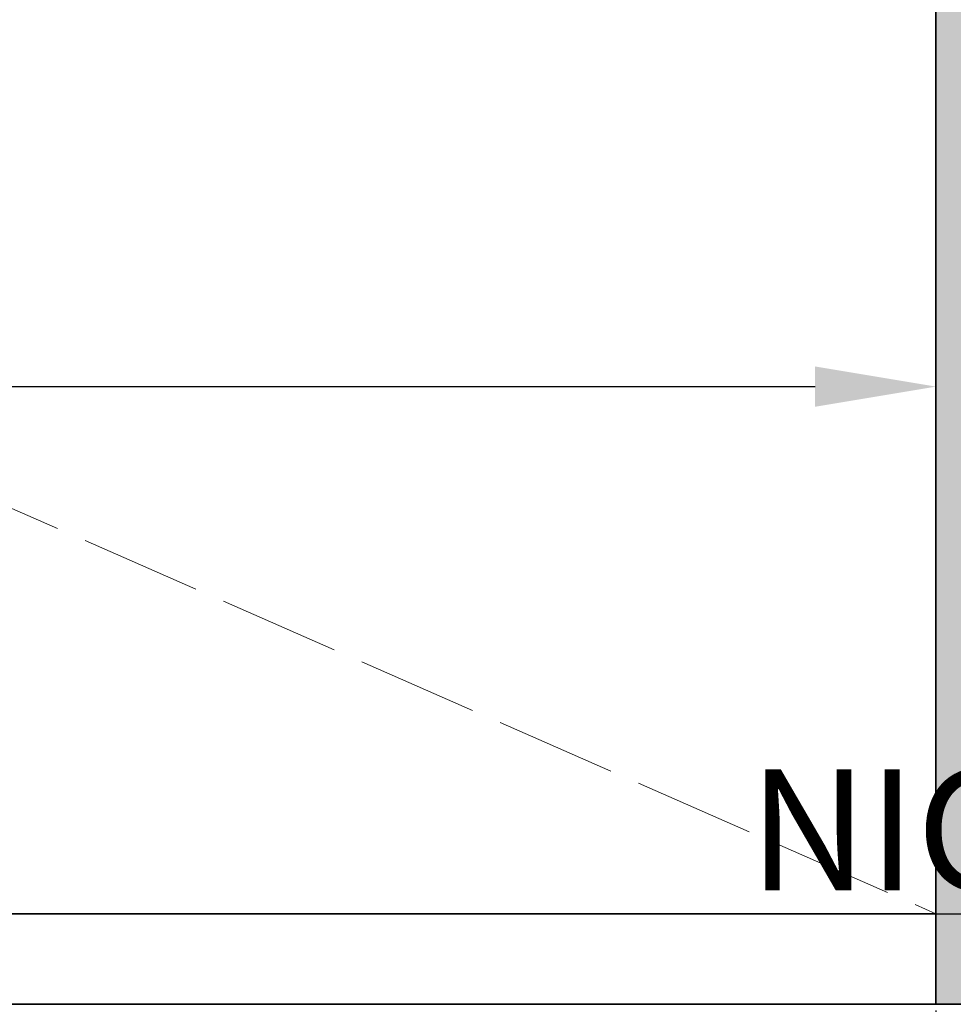
# Model space of a CAD drawing. Units: inches. Extents: x 2083 to 3317, y 1141 to 2115.
# Tile 110 of 256: x 2772 to 2865, y 1263 to 1361. Entities that reach past the tile are written whole.
import ezdxf

# ---------------------------------------------------------------- set-up
doc = ezdxf.new("R2010")
doc.units = ezdxf.units.IN
doc.linetypes.add('ACAD_ISO02W100', pattern=[15, 12, -3])
for name, color, linetype, lineweight in [('A-ANNO-DIMS', 2, 'Continuous', 18), ('A-FLOR-OPEN', 8, 'ACAD_ISO02W100', 13), ('A-WALL', 7, 'Continuous', 35)]:
    doc.layers.add(name, color=color, linetype=linetype, lineweight=lineweight)
doc.layers.add('A-WALL-PATT', color=251, linetype='Continuous', lineweight=13, true_color=0x636466)
doc.styles.get("Standard").update_dxf_attribs({"font": 'arial.ttf'})
doc.dimstyles.new('ISO-25', dxfattribs={"dimtxt": 12, "dimasz": 12, "dimexe": 1.25, "dimexo": 0.625, "dimtad": 1, "dimlunit": 3, "dimtxsty": 'Standard', "dimcen": 2.5, "dimadec": 0, "dimazin": 0, "dimtfac": 1, "dimtmove": 0, "dimatfit": 3, "dimfxl": 1, "dimarcsym": 0})

# ---------------------------------------------------------------- blocks, each defined once
blk = doc.blocks.new('*D10')
at = {"layer": 'A-ANNO-DIMS', "color": 0, "lineweight": -2, "transparency": 16777216}
for p, q in [((2862.96, 1262.636), (2862.96, 1201.384)), ((3126.96, 1262.636), (3126.96, 1201.384)), ((2874.96, 1202.634), (3114.96, 1202.634))]:
    blk.add_line(p, q, dxfattribs=at)
at = {"layer": 'A-ANNO-DIMS', "color": 0, "transparency": 16777216}
for points in [[(2874.96, 1204.634), (2874.96, 1200.634), (2862.96, 1202.634)], [(3114.96, 1204.634), (3114.96, 1200.634), (3126.96, 1202.634)]]:
    blk.add_solid(points, dxfattribs=at)
at = {"layer": 'Defpoints', "color": 0, "transparency": 16777216}
for p in [(2862.96, 1263.261), (3126.96, 1263.261), (3126.96, 1202.634)]:
    blk.add_point(p, dxfattribs=at)
at = {"layer": 'A-ANNO-DIMS', "color": 0, "transparency": 16777216, "insert": (2994.96, 1209.284), "char_height": 12, "attachment_point": 5}
blk.add_mtext("22'", dxfattribs=at)
blk = doc.blocks.new('*D11')
at = {"layer": 'A-ANNO-DIMS', "color": 0, "lineweight": -2, "transparency": 16777216}
for p, q in [((2544.96, 1262.636), (2544.96, 1201.284)), ((2862.96, 1262.636), (2862.96, 1201.284)), ((2556.96, 1202.534), (2850.96, 1202.534))]:
    blk.add_line(p, q, dxfattribs=at)
at = {"layer": 'A-ANNO-DIMS', "color": 0, "transparency": 16777216}
for points in [[(2556.96, 1204.534), (2556.96, 1200.534), (2544.96, 1202.534)], [(2850.96, 1204.534), (2850.96, 1200.534), (2862.96, 1202.534)]]:
    blk.add_solid(points, dxfattribs=at)
at = {"layer": 'Defpoints', "color": 0, "transparency": 16777216}
for p in [(2544.96, 1263.261), (2862.96, 1263.261), (2862.96, 1202.534)]:
    blk.add_point(p, dxfattribs=at)
at = {"layer": 'A-ANNO-DIMS', "color": 0, "transparency": 16777216, "insert": (2703.96, 1209.286), "char_height": 12, "attachment_point": 5}
blk.add_mtext('26\'-6"', dxfattribs=at)
blk = doc.blocks.new('*D26')
at = {"layer": 'A-ANNO-DIMS', "color": 0, "lineweight": -2, "transparency": 16777216}
for p, q in [((3088.986, 1274.915), (3088.986, 1270.952)), ((3111.24, 1274.915), (3111.24, 1270.952)), ((3076.986, 1272.202), (2840.262, 1272.202)), ((3111.24, 1272.202), (3088.986, 1272.202)), ((3123.24, 1272.202), (3135.24, 1272.202))]:
    blk.add_line(p, q, dxfattribs=at)
at = {"layer": 'A-ANNO-DIMS', "color": 0, "transparency": 16777216}
for points in [[(3076.986, 1274.202), (3076.986, 1270.202), (3088.986, 1272.202)], [(3123.24, 1274.202), (3123.24, 1270.202), (3111.24, 1272.202)]]:
    blk.add_solid(points, dxfattribs=at)
at = {"layer": 'Defpoints', "color": 0, "transparency": 16777216}
for p in [(3088.986, 1275.54), (3111.24, 1275.54), (3088.986, 1272.202)]:
    blk.add_point(p, dxfattribs=at)
at = {"layer": 'A-ANNO-DIMS', "color": 0, "transparency": 16777216, "insert": (2952.624, 1279.032), "char_height": 12, "attachment_point": 5}
blk.add_mtext('NIGHTSTAND 1\'-10 1/2" TYP.', dxfattribs=at)
blk = doc.blocks.new('*D66')
at = {"layer": 'A-ANNO-DIMS', "color": 0, "lineweight": -2, "transparency": 16777216}
for p, q in [((2544.96, 1272.886), (2544.96, 1325.861)), ((2862.96, 1272.886), (2862.96, 1325.861)), ((2556.96, 1324.611), (2850.96, 1324.611))]:
    blk.add_line(p, q, dxfattribs=at)
at = {"layer": 'A-ANNO-DIMS', "color": 0, "transparency": 16777216}
for points in [[(2556.96, 1326.611), (2556.96, 1322.611), (2544.96, 1324.611)], [(2850.96, 1326.611), (2850.96, 1322.611), (2862.96, 1324.611)]]:
    blk.add_solid(points, dxfattribs=at)
at = {"layer": 'Defpoints', "color": 0, "transparency": 16777216}
for p in [(2862.96, 1324.611), (2544.96, 1272.261), (2862.96, 1272.261)]:
    blk.add_point(p, dxfattribs=at)
at = {"layer": 'A-ANNO-DIMS', "color": 0, "transparency": 16777216, "insert": (2703.96, 1331.363), "char_height": 12, "attachment_point": 5}
blk.add_mtext('26\'-6"', dxfattribs=at)

msp = doc.modelspace()

# ---------------------------------------------------------------- hatches: boundary and pattern name
at = {"layer": 'A-WALL-PATT'}
h = msp.add_hatch(color=256, dxfattribs=at)
h.dxf.hatch_style = 1
h.paths.add_polyline_path([(3126.96, 2020.761), (2748.96, 2020.761), (2604.96, 2020.761), (2226.96, 2020.761), (2226.96, 1702.761), (2466.96, 1702.761), (2466.96, 1582.761), (2418.96, 1582.761), (2418.96, 1477.761), (2226.96, 1477.761), (2226.96, 1263.261), (2544.96, 1263.261), (2544.96, 1411.761), (2604.96, 1411.761), (2685.96, 1411.761), (2685.96, 1420.761), (2604.96, 1420.761), (2604.96, 1573.761), (2604.96, 1702.761), (2604.96, 2011.761), (2748.96, 2011.761), (2748.96, 1702.761), (2862.96, 1702.761), (2862.96, 1621.761), (2871.96, 1621.761), (2871.96, 1702.761), (2883.96, 1702.761), (2883.96, 1706.939, -0.026459), (2883.96, 1711.761), (2757.96, 1711.761), (2757.96, 1807.761), (2787.96, 1807.761), (2787.96, 1812.261), (2757.96, 1812.261), (2757.96, 2011.761), (2877.96, 2011.761), (2877.96, 1812.261), (2847.96, 1812.261), (2847.96, 1807.761), (2889.836, 1807.761), (2889.836, 1812.261), (2882.46, 1812.261), (2882.46, 2011.761), (3117.96, 2011.761), (3117.96, 1812.261), (2937.836, 1812.261), (2937.836, 1807.761), (2995.71, 1807.761), (2995.71, 1796.118), (3000.21, 1796.118), (3000.21, 1807.761), (3117.96, 1807.761), (3117.96, 1711.761), (3000.21, 1711.761), (3000.21, 1760.118), (2998.573, 1760.118, -0.020711), (2995.71, 1760.118), (2995.71, 1711.761), (2931.96, 1711.761), (2931.96, 1702.761), (3126.96, 1702.761)])
h.paths.add_polyline_path([(2471.46, 2011.761), (2471.46, 1810.011), (2462.717, 1810.011), (2462.717, 1805.511), (2505.96, 1805.511), (2505.96, 1810.011), (2475.96, 1810.011), (2475.96, 2011.761), (2595.96, 2011.761), (2595.96, 1810.011), (2565.96, 1810.011), (2565.96, 1805.511), (2595.96, 1805.511), (2595.96, 1711.761), (2235.96, 1711.761), (2235.96, 1805.511), (2353.71, 1805.511), (2353.71, 1796.054), (2358.21, 1796.054), (2358.21, 1805.511), (2414.717, 1805.511), (2414.717, 1810.011), (2235.96, 1810.011), (2235.96, 2011.761)], flags=16)
h.paths.add_polyline_path([(2270.205, 1994.61), (2270.205, 1970.61), (2246.205, 1970.61), (2246.205, 1994.61)], flags=0)
edge = h.paths.add_edge_path(flags=0)
edge.add_ellipse((2332.027, 1899.798), major_axis=(-3.043, 3.043), ratio=0.168252, start_angle=-161.33217, end_angle=-156.30711, ccw=False)
edge.add_ellipse((2333.082, 1898.744), major_axis=(-1.055, 1.055), ratio=0.453532, start_angle=-123.37102, end_angle=-94.15911)
edge = h.paths.add_edge_path(flags=0)
edge.add_ellipse((2332.027, 1968.876), major_axis=(3.043, 3.043), ratio=0.168252, start_angle=18.66783, end_angle=23.69289)
edge.add_spline(control_points=[(2332.926, 1970.691), (2332.227, 1970.336), (2330.894, 1969.659), (2328.413, 1970.932), (2327.204, 1967.749), (2324.71, 1969.956), (2322.533, 1967.012), (2320.013, 1971.296), (2317.68, 1968.158), (2316.041, 1967.102), (2315.427, 1966.81)], knot_values=[0, 0, 0, 0, 2.267059, 4.324559, 6.685584, 8.878641, 11.121502, 14.300359, 17.755284, 19.732645, 19.732645, 19.732645, 19.732645], degree=3, periodic=0)
edge.add_ellipse((2332.027, 1968.876), major_axis=(3.043, 3.043), ratio=0.168252, start_angle=18.66783, end_angle=23.69289, ccw=False)
edge.add_ellipse((2333.082, 1969.931), major_axis=(1.055, 1.055), ratio=0.453532, start_angle=56.62898, end_angle=85.84089, ccw=False)
edge = h.paths.add_edge_path(flags=0)
edge.add_spline(control_points=[(2296.428, 1967.988), (2293.628, 1965.336), (2287.704, 1959.727), (2299.744, 1949.996), (2294.533, 1935.669), (2290.573, 1920.604), (2293.394, 1909.974), (2296.185, 1904.967)], knot_values=[0.099185, 0.099185, 0.099185, 0.099185, 0.345301, 0.619822, 0.982653, 1.386093, 1.810555, 1.810555, 1.810555, 1.810555], degree=3, periodic=0)
edge.add_spline(control_points=[(2296.185, 1904.967), (2297.384, 1902.619), (2298.001, 1901.949), (2298.553, 1901.468)], knot_values=[0.006246, 0.006246, 0.006246, 0.006246, 0.055476, 0.055476, 0.055476, 0.055476], degree=3, periodic=0)
edge.add_spline(control_points=[(2298.553, 1901.468), (2297.259, 1900.923), (2295.225, 1900.232), (2293.06, 1900.614), (2292.101, 1900.788), (2292.09, 1900.791)], knot_values=[0.312835, 0.312835, 0.312835, 0.312835, 0.40178, 0.474987, 0.475903, 0.475903, 0.475903, 0.475903], degree=3, periodic=0)
edge.add_arc((2292.794, 1904.664), 3.937, 215.4209, 259.69818, ccw=False)
edge.add_spline(control_points=[(2289.585, 1902.382), (2289.477, 1902.535), (2289.368, 1902.688), (2289.261, 1902.841)], knot_values=[0.102872, 0.102872, 0.102872, 0.102872, 0.116896, 0.116896, 0.116896, 0.116896], degree=3, periodic=0)
edge.add_spline(control_points=[(2289.261, 1902.841), (2288.687, 1902.55), (2287.64, 1902.02), (2285.881, 1901.874), (2283.853, 1901.504), (2281.72, 1899.711), (2278.467, 1899.493), (2276.157, 1901.883), (2272.259, 1899.804), (2267.778, 1901.843), (2262.244, 1900.184), (2257.415, 1901.782), (2254.318, 1900.726), (2253.178, 1900.337)], knot_values=[0, 0, 0, 0, 1.907977, 3.477176, 5.261074, 7.972851, 11.680248, 13.717921, 16.939592, 22.789562, 27.502503, 33.595215, 37.145618, 37.145618, 37.145618, 37.145618], degree=3, periodic=0)
edge.add_line((2253.178, 1900.337), (2250.244, 1902.841))
edge.add_line((2250.244, 1902.841), (2250.244, 1965.833))
edge.add_line((2250.244, 1965.833), (2253.178, 1968.337))
edge.add_spline(control_points=[(2253.178, 1968.337), (2254.318, 1967.948), (2257.415, 1966.892), (2262.244, 1968.49), (2267.778, 1966.831), (2271.527, 1968.537), (2273.876, 1967.828), (2274.207, 1967.728)], knot_values=[0, 0, 0, 0, 0.09018, 0.244935, 0.364644, 0.513233, 0.537855, 0.537855, 0.537855, 0.537855], degree=3, periodic=0)
edge.add_arc((2274.353, 1963.793), 3.937, 72.05113, 92.12795, ccw=False)
edge.add_arc((2281.297, 1985.23), 18.596, 252.05113, 288.56572)
edge.add_arc((2292.317, 1956.029), 12.646, 71.02679, 113.77822, ccw=False)
edge = h.paths.add_edge_path(flags=0)
edge.add_spline(control_points=[(2274.899, 1951.856), (2275.066, 1951.617), (2275.233, 1951.377), (2275.398, 1951.136)], knot_values=[1.409916, 1.409916, 1.409916, 1.409916, 1.43159, 1.43159, 1.43159, 1.43159], degree=3, periodic=0)
edge.add_spline(control_points=[(2275.398, 1951.136), (2275.792, 1950.562), (2276.179, 1949.984), (2276.546, 1949.397)], knot_values=[1.358238, 1.358238, 1.358238, 1.358238, 1.409916, 1.409916, 1.409916, 1.409916], degree=3, periodic=0)
edge.add_line((2276.546, 1949.397), (2277.437, 1947.862))
edge.add_spline(control_points=[(2277.437, 1947.862), (2276.304, 1945.673), (2274.64, 1942.427), (2274.632, 1938.094), (2272.799, 1930.852), (2274.356, 1943.897), (2275.948, 1947.923), (2276.546, 1949.397)], knot_values=[0.005632, 0.005632, 0.005632, 0.005632, 0.186014, 0.266002, 0.357087, 0.59639, 0.739732, 0.739732, 0.739732, 0.739732], degree=3, periodic=0)
edge.add_spline(control_points=[(2276.546, 1949.397), (2276.179, 1949.984), (2275.792, 1950.562), (2275.398, 1951.136)], knot_values=[1.358238, 1.358238, 1.358238, 1.358238, 1.409916, 1.409916, 1.409916, 1.409916], degree=3, periodic=0)
edge.add_spline(control_points=[(2275.398, 1951.136), (2274.943, 1950.08), (2274.208, 1948.025), (2273.935, 1944.851), (2272.469, 1937.627), (2273.466, 1945.696), (2274.701, 1951.059), (2274.899, 1951.856)], knot_values=[0.104364, 0.104364, 0.104364, 0.104364, 0.189636, 0.269624, 0.36071, 0.600013, 0.644622, 0.644622, 0.644622, 0.644622], degree=3, periodic=0)
h.paths.add_polyline_path([(2269.168, 1963.128, -0.357527), (2268.171, 1960.976, -0.092561), (2268.171, 1939.436, -0.357527), (2269.168, 1937.285, -0.357527), (2267.016, 1938.282, -0.164785), (2254.686, 1938.282, -0.357527), (2252.534, 1937.285, -0.357527), (2253.531, 1939.436, -0.092561), (2253.531, 1960.976, -0.357527), (2252.534, 1963.128, -0.357527), (2254.686, 1962.131, -0.164785), (2267.016, 1962.131, -0.357527)], flags=0)
h.paths.add_polyline_path([(2248.874, 1967.802), (2248.874, 1957.028), (2249.458, 1957.028), (2249.458, 1911.647), (2248.874, 1911.647), (2248.874, 1900.873), (2246.512, 1900.873, 0.197327), (2244.15, 1902.457), (2244.15, 1966.218, 0.197327), (2246.512, 1967.802)], flags=0)
h.paths.add_polyline_path([(2269.168, 1931.389, -0.357527), (2268.171, 1929.238, -0.092561), (2268.171, 1907.698, -0.357527), (2269.168, 1905.547, -0.357527), (2267.016, 1906.544, -0.164785), (2254.686, 1906.544, -0.357527), (2252.534, 1905.547, -0.357527), (2253.531, 1907.698, -0.092561), (2253.531, 1929.238, -0.357527), (2252.534, 1931.389, -0.357527), (2254.686, 1930.392, -0.164785), (2267.016, 1930.392, -0.357527)], flags=0)
edge = h.paths.add_edge_path(flags=0)
edge.add_spline(control_points=[(2276.197, 1906.724), (2276.168, 1909.029), (2276.114, 1913.372), (2270.598, 1924.925), (2273.905, 1919.013), (2275.922, 1916.262), (2275.475, 1912.402), (2277.258, 1910.381), (2276.696, 1908.225), (2276.646, 1906.813), (2276.618, 1906.008)], knot_values=[0, 0, 0, 0, 8.61026, 16.221274, 18.843057, 23.804898, 27.440828, 29.356102, 31.203478, 33.650687, 33.650687, 33.650687, 33.650687], degree=3, periodic=0)
edge.add_spline(control_points=[(2276.618, 1906.008), (2276.623, 1905.624), (2276.498, 1904.629), (2275.442, 1903.855), (2274.937, 1903.08), (2274.859, 1902.841)], knot_values=[0.156488, 0.156488, 0.156488, 0.156488, 0.184398, 0.231376, 0.250598, 0.250598, 0.250598, 0.250598], degree=3, periodic=0)
edge.add_line((2274.859, 1902.841), (2276.506, 1902.841))
edge.add_spline(control_points=[(2276.506, 1902.841), (2276.788, 1903.085), (2277.665, 1904.125), (2278.25, 1904.341), (2277.654, 1908.527), (2278.156, 1906.228), (2278.1, 1905.286), (2278.847, 1904.069), (2277.857, 1903.415), (2277.874, 1902.991), (2277.904, 1902.841)], knot_values=[0.059574, 0.059574, 0.059574, 0.059574, 0.080753, 0.103741, 0.16972, 0.176036, 0.207137, 0.240474, 0.262341, 0.27366, 0.27366, 0.27366, 0.27366], degree=3, periodic=0)
edge.add_line((2277.904, 1902.841), (2280.03, 1902.841))
edge.add_spline(control_points=[(2280.03, 1902.841), (2279.888, 1903.088), (2279.499, 1903.982), (2280.152, 1905.939), (2278.104, 1909.658), (2279.762, 1907.185), (2280.328, 1904.875), (2280.485, 1903.49), (2281.463, 1903.249), (2281.758, 1902.936), (2281.834, 1902.841)], knot_values=[0.013856, 0.013856, 0.013856, 0.013856, 0.034874, 0.088867, 0.107879, 0.126738, 0.158714, 0.193757, 0.217487, 0.226722, 0.226722, 0.226722, 0.226722], degree=3, periodic=0)
edge.add_spline(control_points=[(2281.834, 1902.841), (2281.788, 1902.827), (2281.647, 1902.783), (2281.396, 1902.859), (2281.088, 1902.985), (2280.721, 1903.061), (2280.333, 1903.026), (2280.125, 1902.899), (2280.03, 1902.841)], knot_values=[0, 0, 0, 0, 0.14413, 0.435517, 0.749276, 1.153046, 1.548371, 1.878348, 1.878348, 1.878348, 1.878348], degree=3, periodic=0)
edge.add_line((2280.03, 1902.841), (2277.904, 1902.841))
edge.add_spline(control_points=[(2277.904, 1902.841), (2277.893, 1902.796), (2277.865, 1902.68), (2277.607, 1902.687), (2277.274, 1902.801), (2276.838, 1902.62), (2276.584, 1902.789), (2276.506, 1902.841)], knot_values=[0, 0, 0, 0, 0.127189, 0.326199, 0.628009, 1.24357, 1.515331, 1.515331, 1.515331, 1.515331], degree=3, periodic=0)
edge.add_line((2276.506, 1902.841), (2274.859, 1902.841))
edge.add_spline(control_points=[(2274.859, 1902.841), (2274.814, 1902.899), (2274.725, 1903.013), (2274.493, 1903.119), (2274.244, 1902.961), (2273.937, 1903.185), (2273.614, 1902.983), (2273.408, 1902.883), (2273.322, 1902.841)], knot_values=[0, 0, 0, 0, 0.21843, 0.436957, 0.687977, 0.990379, 1.398396, 1.69185, 1.69185, 1.69185, 1.69185], degree=3, periodic=0)
edge.add_spline(control_points=[(2273.322, 1902.841), (2273.617, 1903.446), (2274.274, 1904.538), (2276.027, 1904.574), (2276.207, 1906.584), (2276.197, 1906.724)], knot_values=[0.012227, 0.012227, 0.012227, 0.012227, 0.059472, 0.106218, 0.134458, 0.134458, 0.134458, 0.134458], degree=3, periodic=0)
h.paths.add_polyline_path([(2270.776, 1897.79), (2270.776, 1873.79), (2246.776, 1873.79), (2246.776, 1897.79)], flags=0)
h.paths.add_polyline_path([(2353.71, 1760.005), (2353.71, 1760.054), (2358.21, 1760.054, -0.033729)], flags=0)
h.paths.add_polyline_path([(2321.819, 1737.529), (2341.995, 1737.529, -0.414214), (2343.203, 1736.321), (2343.203, 1721.021, -0.414214), (2341.995, 1719.813), (2321.819, 1719.813, -0.414214), (2320.611, 1721.021), (2320.611, 1736.321, -0.414214)], flags=0)
h.paths.add_polyline_path([(2324.235, 1736.321), (2339.579, 1736.321, -0.414214), (2341.995, 1733.905), (2341.995, 1725.45, -0.414214), (2339.579, 1723.034), (2333.681, 1723.034), (2333.845, 1722.045, -0.870646), (2335.425, 1721.826, -0.767327), (2333.923, 1721.423), (2331.291, 1721.423, -0.767327), (2329.788, 1721.826, -0.870646), (2331.368, 1722.045), (2331.533, 1723.034), (2324.235, 1723.034, -0.414214), (2321.819, 1725.45), (2321.819, 1733.905, -0.414214)], flags=0)
h.paths.add_polyline_path([(2570.484, 1928.615), (2589.684, 1928.615), (2590.169, 1928.615), (2590.169, 1904.993), (2570.484, 1904.993)], flags=0)
h.paths.add_polyline_path([(2574.447, 1927.264, -1), (2572.829, 1927.264, -1)], flags=0)
h.paths.add_polyline_path([(2573.09, 1926.941), (2573.925, 1927.776), (2574.148, 1927.553), (2573.313, 1926.718)], flags=0)
h.paths.add_polyline_path([(2578.779, 1919.73, -1), (2571.592, 1919.73, -1)], flags=0)
h.paths.add_polyline_path([(2578.385, 1919.73, -1), (2571.985, 1919.73, -1)], flags=0)
h.paths.add_polyline_path([(2331.596, 1729.476, -1), (2333.618, 1729.476, -1)], flags=0)
h.paths.add_polyline_path([(2578.034, 1927.264, -1), (2576.416, 1927.264, -1)], flags=0)
h.paths.add_polyline_path([(2576.689, 1927.531), (2576.912, 1927.754), (2577.747, 1926.919), (2577.524, 1926.696)], flags=0)
h.paths.add_polyline_path([(2578.139, 1909.86, -1), (2572.232, 1909.86, -1)], flags=0)
h.paths.add_polyline_path([(2577.745, 1909.86, -1), (2572.625, 1909.86, -1)], flags=0)
h.paths.add_polyline_path([(2583.798, 1927.264, -1), (2582.179, 1927.264, -1)], flags=0)
h.paths.add_polyline_path([(2582.719, 1927.754), (2583.554, 1926.919), (2583.331, 1926.696), (2582.496, 1927.531)], flags=0)
h.paths.add_polyline_path([(2582.496, 1927.531), (2582.719, 1927.754), (2583.554, 1926.919), (2583.331, 1926.696)], flags=0)
h.paths.add_polyline_path([(2587.739, 1920.53, -1), (2581.832, 1920.53, -1)], flags=0)
h.paths.add_polyline_path([(2587.345, 1920.53, -1), (2582.225, 1920.53, -1)], flags=0)
h.paths.add_polyline_path([(2587.385, 1927.264, -1), (2585.766, 1927.264, -1)], flags=0)
h.paths.add_polyline_path([(2586.082, 1926.98), (2586.917, 1927.815), (2587.14, 1927.593), (2586.305, 1926.758)], flags=0)
h.paths.add_polyline_path([(2588.379, 1910.66, -1), (2581.192, 1910.66, -1)], flags=0)
h.paths.add_polyline_path([(2587.985, 1910.66, -1), (2581.585, 1910.66, -1)], flags=0)
h.paths.add_polyline_path([(2417.168, 1729.478), (2437.344, 1729.478, -0.414214), (2438.552, 1728.27), (2438.552, 1712.969, -0.414214), (2437.344, 1711.761), (2417.168, 1711.761, -0.414214), (2415.96, 1712.969), (2415.96, 1728.27, -0.414214)], flags=0)
h.paths.add_polyline_path([(2419.584, 1728.27), (2434.928, 1728.27, -0.414214), (2437.344, 1725.854), (2437.344, 1717.398, -0.414214), (2434.928, 1714.983), (2429.029, 1714.983), (2429.194, 1713.994, -0.870646), (2430.774, 1713.775, -0.767327), (2429.271, 1713.372), (2426.64, 1713.372, -0.767327), (2425.137, 1713.775, -0.870646), (2426.717, 1713.994), (2426.882, 1714.983), (2419.584, 1714.983, -0.414214), (2417.168, 1717.398), (2417.168, 1725.854, -0.414214)], flags=0)
h.paths.add_polyline_path([(2419.584, 1728.27), (2434.928, 1728.27, -0.414214), (2437.344, 1725.854), (2437.344, 1717.398, -0.414214), (2434.928, 1714.983), (2429.029, 1714.983), (2428.358, 1719.009), (2427.553, 1719.009), (2426.882, 1714.983), (2419.584, 1714.983, -0.414214), (2417.168, 1717.398), (2417.168, 1725.854, -0.414214)], flags=0)
h.paths.add_polyline_path([(2426.944, 1721.425, -1), (2428.967, 1721.425, -1)], flags=0)
h.paths.add_polyline_path([(2475.96, 1702.761), (2595.96, 1702.761), (2595.96, 1582.761), (2475.96, 1582.761)], flags=16)
h.paths.add_polyline_path([(2427.96, 1573.761), (2595.96, 1573.761), (2595.96, 1468.761), (2595.96, 1420.761), (2384.46, 1420.761), (2384.46, 1468.761), (2427.96, 1468.761)], flags=16)
h.paths.add_polyline_path([(2379.96, 1468.761), (2379.96, 1420.761), (2235.96, 1420.761), (2235.96, 1468.761)], flags=16)
h.paths.add_polyline_path([(2317.816, 1466.696), (2337.992, 1466.696, -0.414214), (2339.2, 1465.488), (2339.2, 1450.187, -0.414214), (2337.992, 1448.979), (2317.816, 1448.979, -0.414214), (2316.608, 1450.187), (2316.608, 1465.488, -0.414214)], flags=0)
h.paths.add_polyline_path([(2320.232, 1465.488), (2335.576, 1465.488, -0.414214), (2337.992, 1463.072), (2337.992, 1454.616, -0.414214), (2335.576, 1452.2), (2329.677, 1452.2), (2329.842, 1451.212, -0.870646), (2331.422, 1450.992, -0.767327), (2329.92, 1450.59), (2327.288, 1450.59, -0.767327), (2325.785, 1450.992, -0.870646), (2327.365, 1451.212), (2327.53, 1452.2), (2320.232, 1452.2, -0.414214), (2317.816, 1454.616), (2317.816, 1463.072, -0.414214)], flags=0)
h.paths.add_polyline_path([(2320.232, 1465.488), (2335.576, 1465.488, -0.414214), (2337.992, 1463.072), (2337.992, 1454.616, -0.414214), (2335.576, 1452.2), (2329.677, 1452.2), (2329.006, 1456.227), (2328.201, 1456.227), (2327.53, 1452.2), (2320.232, 1452.2, -0.414214), (2317.816, 1454.616), (2317.816, 1463.072, -0.414214)], flags=0)
h.paths.add_polyline_path([(2327.593, 1458.643, -1), (2329.615, 1458.643, -1)], flags=0)
h.paths.add_polyline_path([(2244.412, 1433.34), (2241.921, 1433.34, -0.414214), (2240.018, 1435.244), (2240.018, 1440.953, -0.414211), (2241.921, 1442.856), (2244.412, 1442.856, -1.976472)], flags=0)
h.paths.add_polyline_path([(2245.357, 1434.398, -0.414214), (2245.357, 1441.799, -2.144098)], flags=0)
h.paths.add_polyline_path([(2535.96, 1416.261), (2535.96, 1272.261), (2235.96, 1272.261), (2235.96, 1416.261)], flags=16)
h.paths.add_polyline_path([(2260.12, 1384.293), (2260.12, 1362.039), (2237.865, 1362.039), (2237.865, 1384.293)], flags=0)
edge = h.paths.add_edge_path(flags=0)
edge.add_line((2318.252, 1362.093), (2318.146, 1362.001))
edge.add_ellipse((2317.445, 1360.431), major_axis=(2.822, 2.822), ratio=0.168252, start_angle=18.66783, end_angle=20.94813, ccw=False)
edge.add_ellipse((2318.423, 1361.409), major_axis=(0.978, 0.978), ratio=0.453532, start_angle=56.62898, end_angle=70.2262, ccw=False)
edge = h.paths.add_edge_path(flags=0)
edge.add_line((2319.107, 1295.571), (2319.015, 1295.677))
edge.add_ellipse((2317.445, 1296.378), major_axis=(-2.822, 2.822), ratio=0.168252, start_angle=-161.33217, end_angle=-159.05187, ccw=False)
edge.add_ellipse((2318.423, 1295.4), major_axis=(-0.978, 0.978), ratio=0.453532, start_angle=-123.37102, end_angle=-109.7738)
edge = h.paths.add_edge_path(flags=0)
edge.add_spline(control_points=[(2284.21, 1301.17), (2284.581, 1300.445), (2284.891, 1299.892), (2285.16, 1299.461)], knot_values=[0.039066, 0.039066, 0.039066, 0.039066, 0.055476, 0.055476, 0.055476, 0.055476], degree=3, periodic=0)
edge.add_line((2285.16, 1299.461), (2284.21, 1301.17))
edge = h.paths.add_edge_path(flags=0)
edge.add_line((2280.412, 1297.298), (2283.37, 1297.036))
edge.add_line((2283.37, 1297.036), (2286.406, 1297.926))
edge.add_spline(control_points=[(2286.406, 1297.926), (2285.305, 1297.463), (2284.345, 1297.129), (2283.37, 1297.036)], knot_values=[0.394369, 0.394369, 0.394369, 0.394369, 0.475903, 0.475903, 0.475903, 0.475903], degree=3, periodic=0)
edge.add_spline(control_points=[(2283.37, 1297.036), (2283.281, 1297.028), (2282.316, 1296.957), (2281.313, 1297.134), (2280.423, 1297.296), (2280.412, 1297.298)], knot_values=[0.312835, 0.312835, 0.312835, 0.312835, 0.320246, 0.393453, 0.394369, 0.394369, 0.394369, 0.394369], degree=3, periodic=0)
edge = h.paths.add_edge_path(flags=0)
edge.add_line((2284.436, 1359.607), (2280.446, 1355.328))
edge.add_line((2280.446, 1355.328), (2279.58, 1351.018))
edge.add_line((2279.58, 1351.018), (2282.413, 1346.58))
edge.add_spline(control_points=[(2282.413, 1346.58), (2283.153, 1345.589), (2284.253, 1344.029), (2284.801, 1342.387), (2284.935, 1341.806)], knot_values=[1.240098, 1.240098, 1.240098, 1.240098, 1.332892, 1.382712, 1.382712, 1.382712, 1.382712], degree=3, periodic=0)
edge.add_spline(control_points=[(2284.935, 1341.806), (2285.319, 1340.141), (2285.233, 1338.409), (2284.91, 1336.654)], knot_values=[1.097484, 1.097484, 1.097484, 1.097484, 1.240098, 1.240098, 1.240098, 1.240098], degree=3, periodic=0)
edge.add_spline(control_points=[(2284.91, 1336.654), (2284.587, 1334.899), (2284.027, 1333.12), (2283.463, 1331.361)], knot_values=[0.95487, 0.95487, 0.95487, 0.95487, 1.097484, 1.097484, 1.097484, 1.097484], degree=3, periodic=0)
edge.add_line((2283.463, 1331.361), (2281.89, 1326.153))
edge.add_line((2281.89, 1326.153), (2280.756, 1321.056))
edge.add_line((2280.756, 1321.056), (2280.299, 1316.002))
edge.add_line((2280.299, 1316.002), (2280.716, 1310.95))
edge.add_line((2280.716, 1310.95), (2282.028, 1305.972))
edge.add_line((2282.028, 1305.972), (2284.21, 1301.17))
edge.add_spline(control_points=[(2284.21, 1301.17), (2283.341, 1302.73), (2282.612, 1304.336), (2282.028, 1305.972)], knot_values=[0.099185, 0.099185, 0.099185, 0.099185, 0.241799, 0.241799, 0.241799, 0.241799], degree=3, periodic=0)
edge.add_spline(control_points=[(2282.028, 1305.972), (2281.444, 1307.608), (2281.005, 1309.273), (2280.716, 1310.95)], knot_values=[0.241799, 0.241799, 0.241799, 0.241799, 0.384413, 0.384413, 0.384413, 0.384413], degree=3, periodic=0)
edge.add_spline(control_points=[(2280.716, 1310.95), (2280.433, 1312.588), (2280.289, 1314.277), (2280.299, 1315.962), (2280.299, 1316.002)], knot_values=[0.384413, 0.384413, 0.384413, 0.384413, 0.523647, 0.527028, 0.527028, 0.527028, 0.527028], degree=3, periodic=0)
edge.add_spline(control_points=[(2280.299, 1316.002), (2280.312, 1317.687), (2280.478, 1319.368), (2280.756, 1321.056)], knot_values=[0.527028, 0.527028, 0.527028, 0.527028, 0.669642, 0.669642, 0.669642, 0.669642], degree=3, periodic=0)
edge.add_spline(control_points=[(2280.756, 1321.056), (2281.035, 1322.744), (2281.426, 1324.44), (2281.89, 1326.153)], knot_values=[0.669642, 0.669642, 0.669642, 0.669642, 0.812256, 0.812256, 0.812256, 0.812256], degree=3, periodic=0)
edge.add_spline(control_points=[(2281.89, 1326.153), (2282.264, 1327.533), (2282.788, 1329.262), (2283.353, 1331.018), (2283.463, 1331.361)], knot_values=[0.812256, 0.812256, 0.812256, 0.812256, 0.927087, 0.95487, 0.95487, 0.95487, 0.95487], degree=3, periodic=0)
edge.add_line((2283.463, 1331.361), (2284.91, 1336.654))
edge.add_line((2284.91, 1336.654), (2284.935, 1341.806))
edge.add_line((2284.935, 1341.806), (2282.413, 1346.58))
edge.add_spline(control_points=[(2282.413, 1346.58), (2281.275, 1348.104), (2280.078, 1349.57), (2279.58, 1351.018)], knot_values=[1.382712, 1.382712, 1.382712, 1.382712, 1.525326, 1.525326, 1.525326, 1.525326], degree=3, periodic=0)
edge.add_spline(control_points=[(2279.58, 1351.018), (2279.443, 1351.415), (2279.136, 1352.857), (2279.735, 1354.29), (2280.446, 1355.328)], knot_values=[1.525326, 1.525326, 1.525326, 1.525326, 1.564439, 1.667941, 1.667941, 1.667941, 1.667941], degree=3, periodic=0)
edge.add_spline(control_points=[(2280.446, 1355.328), (2281.426, 1356.758), (2282.931, 1358.183), (2284.436, 1359.607)], knot_values=[1.667941, 1.667941, 1.667941, 1.667941, 1.810555, 1.810555, 1.810555, 1.810555], degree=3, periodic=0)
edge.add_arc((2280.623, 1348.518), 11.726, 71.02679, 113.77822)
edge.add_arc((2270.405, 1375.595), 17.244, 252.05113, 288.56572, ccw=False)
edge.add_arc((2263.966, 1355.718), 3.651, 72.05113, 92.12795)
edge.add_arc((2263.966, 1355.718), 3.651, 92.12795, 177.98513)
edge.add_spline(control_points=[(2260.318, 1355.846), (2260.26, 1354.221), (2260.551, 1350.187), (2262.999, 1346.766), (2264.473, 1344.649)], knot_values=[1.43159, 1.43159, 1.43159, 1.43159, 1.564144, 1.770695, 1.770695, 1.770695, 1.770695], degree=3, periodic=0)
edge.add_line((2264.473, 1344.649), (2264.936, 1343.983))
edge.add_spline(control_points=[(2263.801, 1340.248), (2263.843, 1340.514), (2264.067, 1341.756), (2264.513, 1343.002), (2264.935, 1343.981)], knot_values=[0.53657, 0.53657, 0.53657, 0.53657, 0.559349, 0.644622, 0.644622, 0.644622, 0.644622], degree=3, periodic=0)
edge.add_spline(control_points=[(2264.935, 1343.981), (2265.118, 1343.715), (2265.299, 1343.448), (2265.477, 1343.179)], knot_values=[1.384077, 1.384077, 1.384077, 1.384077, 1.409916, 1.409916, 1.409916, 1.409916], degree=3, periodic=0)
edge.add_spline(control_points=[(2265.477, 1343.179), (2265.655, 1342.911), (2265.829, 1342.641), (2265.999, 1342.369)], knot_values=[1.358238, 1.358238, 1.358238, 1.358238, 1.384077, 1.384077, 1.384077, 1.384077], degree=3, periodic=0)
edge.add_line((2265.999, 1342.369), (2266.826, 1340.946))
edge.add_spline(control_points=[(2266.826, 1340.946), (2268.894, 1337.09), (2271.398, 1325.843), (2270.516, 1310.569), (2275.919, 1301.861), (2277.79, 1299.199)], knot_values=[0.116896, 0.116896, 0.116896, 0.116896, 0.472987, 1.050969, 1.313793, 1.313793, 1.313793, 1.313793], degree=3, periodic=0)
edge.add_spline(control_points=[(2277.79, 1299.199), (2277.839, 1299.128), (2277.889, 1299.057), (2277.94, 1298.987)], knot_values=[0.109884, 0.109884, 0.109884, 0.109884, 0.116896, 0.116896, 0.116896, 0.116896], degree=3, periodic=0)
edge.add_line((2277.94, 1298.987), (2277.789, 1299.199))
edge.add_spline(control_points=[(2277.789, 1299.199), (2277.257, 1298.929), (2276.286, 1298.438), (2275.039, 1298.334), (2274.383, 1298.239), (2274.215, 1298.209)], knot_values=[33.12187, 33.12187, 33.12187, 33.12187, 35.029056, 36.598255, 37.144827, 37.144827, 37.144827, 37.144827], degree=3, periodic=0)
edge.add_line((2274.215, 1298.209), (2273.073, 1297.893))
edge.add_spline(control_points=[(2273.073, 1297.893), (2272.323, 1297.58), (2271.039, 1296.511), (2269.248, 1296.226), (2268.423, 1296.375)], knot_values=[26.532584, 26.532584, 26.532584, 26.532584, 29.198919, 31.839101, 31.839101, 31.839101, 31.839101], degree=3, periodic=0)
edge.add_line((2268.423, 1296.375), (2263.879, 1297.458))
edge.add_spline(control_points=[(2263.879, 1297.458), (2263.556, 1297.359), (2261.86, 1296.839), (2260.239, 1297.282), (2258.933, 1297.516)], knot_values=[15.919551, 15.919551, 15.919551, 15.919551, 16.939592, 21.226067, 21.226067, 21.226067, 21.226067], degree=3, periodic=0)
edge.add_line((2258.933, 1297.516), (2254.055, 1297.329))
edge.add_spline(control_points=[(2254.055, 1297.329), (2253.756, 1297.296), (2252.114, 1297.165), (2250.462, 1297.544), (2249.13, 1297.668)], knot_values=[5.306517, 5.306517, 5.306517, 5.306517, 6.276435, 10.613034, 10.613034, 10.613034, 10.613034], degree=3, periodic=0)
edge.add_line((2249.13, 1297.668), (2244.332, 1296.878))
edge.add_line((2244.332, 1296.878), (2241.611, 1299.199))
edge.add_line((2241.611, 1299.199), (2241.611, 1357.609))
edge.add_line((2241.611, 1357.609), (2244.332, 1359.931))
edge.add_line((2244.332, 1359.931), (2252.729, 1359.543))
edge.add_spline(control_points=[(2252.729, 1359.543), (2252.871, 1359.546), (2253.306, 1359.548), (2253.74, 1359.514), (2254.032, 1359.482)], knot_values=[0.233291, 0.233291, 0.233291, 0.233291, 0.244935, 0.268927, 0.268927, 0.268927, 0.268927], degree=3, periodic=0)
edge.add_line((2254.032, 1359.482), (2259.587, 1359.416))
edge.add_spline(control_points=[(2259.587, 1359.416), (2260.677, 1359.629), (2262.073, 1359.897), (2263.524, 1359.459), (2263.83, 1359.366)], knot_values=[0.422516, 0.422516, 0.422516, 0.422516, 0.513233, 0.537855, 0.537855, 0.537855, 0.537855], degree=3, periodic=0)
edge.add_arc((2263.966, 1355.718), 3.651, 72.05113, 92.12795, ccw=False)
edge.add_arc((2270.405, 1375.595), 17.244, 252.05113, 288.56572)
edge.add_arc((2280.623, 1348.518), 11.726, 71.02679, 113.77822, ccw=False)
h.paths.add_polyline_path([(2240.341, 1359.435), (2240.341, 1349.444), (2240.882, 1349.444), (2240.882, 1307.365), (2240.341, 1307.365), (2240.341, 1297.374), (2238.15, 1297.374, 0.197327), (2235.96, 1298.843), (2235.96, 1357.966, 0.197327), (2238.15, 1359.435)], flags=0)
h.paths.add_polyline_path([(2259.158, 1355.101, -0.357527), (2258.233, 1353.106, -0.092561), (2258.233, 1333.133, -0.357527), (2259.158, 1331.138, -0.357527), (2257.163, 1332.062, -0.164785), (2245.729, 1332.062, -0.357527), (2243.735, 1331.138, -0.357527), (2244.659, 1333.133, -0.092561), (2244.659, 1353.106, -0.357527), (2243.735, 1355.101, -0.357527), (2245.729, 1354.176, -0.164785), (2257.163, 1354.176, -0.357527)], flags=0)
edge = h.paths.add_edge_path(flags=0)
edge.add_line((2265.999, 1342.369), (2266.826, 1340.946))
edge.add_line((2266.826, 1340.946), (2265.308, 1337.814))
edge.add_line((2265.308, 1337.814), (2264.358, 1334.653))
edge.add_line((2264.358, 1334.653), (2264.262, 1333.8))
edge.add_spline(control_points=[(2264.262, 1333.8), (2264.208, 1333.187), (2264.162, 1332.366), (2264.007, 1331.414), (2263.969, 1331.202)], knot_values=[0.464444, 0.464444, 0.464444, 0.464444, 0.516691, 0.531608, 0.531608, 0.531608, 0.531608], degree=3, periodic=0)
edge.add_spline(control_points=[(2263.969, 1331.202), (2263.775, 1330.119), (2263.424, 1328.791), (2263.257, 1328.531), (2263.234, 1328.515)], knot_values=[0.372682, 0.372682, 0.372682, 0.372682, 0.44885, 0.464444, 0.464444, 0.464444, 0.464444], degree=3, periodic=0)
edge.add_spline(control_points=[(2263.234, 1328.515), (2263.096, 1328.42), (2263.131, 1329.301), (2263.275, 1330.616)], knot_values=[0.280919, 0.280919, 0.280919, 0.280919, 0.372682, 0.372682, 0.372682, 0.372682], degree=3, periodic=0)
edge.add_spline(control_points=[(2263.275, 1330.616), (2263.419, 1331.93), (2263.672, 1333.677), (2263.97, 1335.315)], knot_values=[0.189157, 0.189157, 0.189157, 0.189157, 0.280919, 0.280919, 0.280919, 0.280919], degree=3, periodic=0)
edge.add_spline(control_points=[(2263.97, 1335.315), (2264.1, 1336.032), (2264.419, 1337.622), (2264.755, 1338.864), (2264.947, 1339.491)], knot_values=[0.097394, 0.097394, 0.097394, 0.097394, 0.137578, 0.189157, 0.189157, 0.189157, 0.189157], degree=3, periodic=0)
edge.add_spline(control_points=[(2264.947, 1339.491), (2265.29, 1340.606), (2265.644, 1341.494), (2265.999, 1342.369)], knot_values=[0.005632, 0.005632, 0.005632, 0.005632, 0.097394, 0.097394, 0.097394, 0.097394], degree=3, periodic=0)
h.paths.add_polyline_path([(2259.158, 1325.671, -0.357527), (2258.233, 1323.676, -0.092561), (2258.233, 1303.703, -0.357527), (2259.158, 1301.708, -0.357527), (2257.163, 1302.633, -0.164785), (2245.729, 1302.633, -0.357527), (2243.735, 1301.708, -0.357527), (2244.659, 1303.703, -0.092561), (2244.659, 1323.676, -0.357527), (2243.735, 1325.671, -0.357527), (2245.729, 1324.747, -0.164785), (2257.163, 1324.747, -0.357527)], flags=0)
edge = h.paths.add_edge_path(flags=0)
edge.add_spline(control_points=[(2261.709, 1317.311), (2261.679, 1317.418), (2261.762, 1317.389), (2262.491, 1316.09), (2262.962, 1315.301)], knot_values=[14.955861, 14.955861, 14.955861, 14.955861, 16.221274, 18.694826, 18.694826, 18.694826, 18.694826], degree=3, periodic=0)
edge.add_spline(control_points=[(2262.962, 1315.301), (2262.99, 1315.254), (2263.702, 1314.067), (2264.349, 1313.127), (2264.73, 1312.164)], knot_values=[18.694826, 18.694826, 18.694826, 18.694826, 18.843057, 22.433791, 22.433791, 22.433791, 22.433791], degree=3, periodic=0)
edge.add_spline(control_points=[(2264.73, 1312.164), (2264.876, 1311.796), (2265.177, 1310.77), (2265.143, 1309.559), (2265.248, 1308.824)], knot_values=[22.433791, 22.433791, 22.433791, 22.433791, 23.804898, 26.172756, 26.172756, 26.172756, 26.172756], degree=3, periodic=0)
edge.add_line((2265.248, 1308.824), (2265.851, 1307.172))
edge.add_spline(control_points=[(2265.851, 1307.172), (2266.065, 1306.822), (2266.384, 1306.332), (2266.424, 1305.781), (2266.42, 1305.611)], knot_values=[28.062562, 28.062562, 28.062562, 28.062562, 29.356102, 29.911721, 29.911721, 29.911721, 29.911721], degree=3, periodic=0)
edge.add_spline(control_points=[(2266.42, 1305.611), (2266.416, 1305.433), (2266.394, 1305.25), (2266.365, 1305.066)], knot_values=[29.911721, 29.911721, 29.911721, 29.911721, 30.497837, 30.497837, 30.497837, 30.497837], degree=3, periodic=0)
edge.add_line((2266.365, 1305.066), (2266.066, 1302.136))
edge.add_spline(control_points=[(2266.066, 1302.136), (2266.071, 1301.78), (2265.998, 1301.2), (2265.663, 1300.759), (2265.509, 1300.586)], knot_values=[0.156488, 0.156488, 0.156488, 0.156488, 0.184398, 0.203543, 0.203543, 0.203543, 0.203543], degree=3, periodic=0)
edge.add_line((2265.509, 1300.586), (2264.435, 1299.199))
edge.add_line((2264.435, 1299.199), (2265.962, 1299.199))
edge.add_line((2265.962, 1299.199), (2267.336, 1301.175))
edge.add_line((2267.336, 1301.175), (2267.312, 1301.986))
edge.add_spline(control_points=[(2267.312, 1301.986), (2267.261, 1302.862), (2267.16, 1303.737), (2267.271, 1303.326)], knot_values=[0.126229, 0.126229, 0.126229, 0.126229, 0.166617, 0.166617, 0.166617, 0.166617], degree=3, periodic=0)
edge.add_spline(control_points=[(2267.271, 1303.326), (2267.28, 1303.294), (2267.31, 1303.175), (2267.373, 1302.884), (2267.406, 1302.683), (2267.418, 1302.601)], knot_values=[0.166617, 0.166617, 0.166617, 0.166617, 0.16972, 0.176036, 0.180765, 0.180765, 0.180765, 0.180765], degree=3, periodic=0)
edge.add_spline(control_points=[(2267.744, 1300.988), (2267.688, 1301.151), (2267.481, 1301.657), (2267.484, 1302.145), (2267.418, 1302.601)], knot_values=[0.180765, 0.180765, 0.180765, 0.180765, 0.193767, 0.220139, 0.220139, 0.220139, 0.220139], degree=3, periodic=0)
edge.add_line((2267.418, 1302.601), (2267.744, 1300.988))
edge.add_spline(control_points=[(2267.744, 1300.988), (2267.832, 1300.732), (2267.932, 1300.31), (2267.555, 1299.975), (2267.429, 1299.829)], knot_values=[0.220139, 0.220139, 0.220139, 0.220139, 0.240474, 0.25489, 0.25489, 0.25489, 0.25489], degree=3, periodic=0)
edge.add_line((2267.429, 1299.829), (2267.258, 1299.199))
edge.add_line((2267.258, 1299.199), (2269.23, 1299.199))
edge.add_spline(control_points=[(2269.23, 1299.199), (2269.099, 1299.429), (2268.843, 1300.016), (2269.012, 1300.916), (2268.947, 1301.661)], knot_values=[0.013856, 0.013856, 0.013856, 0.013856, 0.034874, 0.067073, 0.067073, 0.067073, 0.067073], degree=3, periodic=0)
edge.add_line((2268.947, 1301.661), (2268.432, 1303.603))
edge.add_spline(control_points=[(2268.432, 1303.603), (2268.176, 1304.192), (2267.596, 1305.251), (2268.041, 1304.623), (2268.251, 1304.282)], knot_values=[0.090155, 0.090155, 0.090155, 0.090155, 0.107879, 0.120289, 0.120289, 0.120289, 0.120289], degree=3, periodic=0)
edge.add_spline(control_points=[(2268.251, 1304.282), (2268.361, 1304.105), (2269.058, 1302.918), (2269.383, 1301.59), (2269.521, 1300.776), (2269.575, 1300.556)], knot_values=[0.120289, 0.120289, 0.120289, 0.120289, 0.126738, 0.158714, 0.173506, 0.173506, 0.173506, 0.173506], degree=3, periodic=0)
edge.add_line((2269.575, 1300.556), (2270.686, 1299.421))
edge.add_spline(control_points=[(2270.686, 1299.421), (2270.767, 1299.357), (2270.838, 1299.281), (2270.903, 1299.199)], knot_values=[0.21816, 0.21816, 0.21816, 0.21816, 0.226722, 0.226722, 0.226722, 0.226722], degree=3, periodic=0)
edge.add_line((2270.937, 1299.193), (2270.903, 1299.199))
edge.add_spline(control_points=[(2270.903, 1299.199), (2270.86, 1299.186), (2270.73, 1299.146), (2270.496, 1299.216), (2270.272, 1299.308), (2270.121, 1299.348), (2270.063, 1299.36)], knot_values=[0.939174, 0.939174, 0.939174, 0.939174, 1.083304, 1.374691, 1.68845, 1.878348, 1.878348, 1.878348, 1.878348], degree=3, periodic=0)
edge.add_line((2270.063, 1299.36), (2269.23, 1299.199))
edge.add_line((2269.23, 1299.199), (2267.258, 1299.199))
edge.add_spline(control_points=[(2267.258, 1299.199), (2267.248, 1299.157), (2267.223, 1299.05), (2266.984, 1299.057), (2266.809, 1299.116), (2266.677, 1299.109), (2266.637, 1299.105)], knot_values=[0.757665, 0.757665, 0.757665, 0.757665, 0.884854, 1.083864, 1.385675, 1.515331, 1.515331, 1.515331, 1.515331], degree=3, periodic=0)
edge.add_spline(control_points=[(2266.637, 1299.105), (2266.485, 1299.089), (2266.236, 1299.017), (2266.035, 1299.151), (2265.962, 1299.199)], knot_values=[0, 0, 0, 0, 0.485905, 0.757665, 0.757665, 0.757665, 0.757665], degree=3, periodic=0)
edge.add_line((2265.962, 1299.199), (2264.435, 1299.199))
edge.add_line((2264.435, 1299.199), (2263.858, 1299.367))
edge.add_spline(control_points=[(2263.858, 1299.367), (2263.819, 1299.371), (2263.78, 1299.386), (2263.74, 1299.402)], knot_values=[0.845925, 0.845925, 0.845925, 0.845925, 0.978627, 0.978627, 0.978627, 0.978627], degree=3, periodic=0)
edge.add_line((2263.722, 1299.396), (2263.01, 1299.199))
edge.add_spline(control_points=[(2263.01, 1299.199), (2263.246, 1299.683), (2263.506, 1300.128), (2263.873, 1300.408)], knot_values=[0.012227, 0.012227, 0.012227, 0.012227, 0.052971, 0.052971, 0.052971, 0.052971], degree=3, periodic=0)
edge.add_spline(control_points=[(2263.873, 1300.408), (2263.932, 1300.453), (2264.084, 1300.553), (2264.255, 1300.624), (2264.36, 1300.665)], knot_values=[0.052971, 0.052971, 0.052971, 0.052971, 0.059472, 0.069086, 0.069086, 0.069086, 0.069086], degree=3, periodic=0)
edge.add_line((2264.36, 1300.665), (2265.142, 1301.078))
edge.add_line((2265.142, 1301.078), (2265.676, 1302.8))
edge.add_line((2265.676, 1302.8), (2265.541, 1305.704))
edge.add_line((2265.541, 1305.704), (2264.803, 1309.328))
edge.add_line((2264.803, 1309.328), (2263.041, 1314.092))
edge.add_spline(control_points=[(2263.041, 1314.092), (2262.384, 1315.671), (2261.796, 1316.998), (2261.709, 1317.311)], knot_values=[11.216896, 11.216896, 11.216896, 11.216896, 14.955861, 14.955861, 14.955861, 14.955861], degree=3, periodic=0)
h.paths.add_polyline_path([(2871.96, 1416.261), (2895.91, 1416.261), (2895.91, 1420.761), (2871.96, 1420.761), (2871.96, 1501.761), (2862.96, 1501.761), (2862.96, 1420.761), (2805.96, 1420.761), (2805.96, 1411.761), (2862.96, 1411.761), (2862.96, 1263.261), (3126.96, 1263.261), (3126.96, 1411.761), (3126.96, 1486.761), (2943.96, 1486.761), (2943.96, 1477.761), (2967.86, 1477.761), (2967.86, 1420.761), (2943.91, 1420.761), (2943.91, 1416.261), (3117.96, 1416.261), (3117.96, 1420.761), (2972.36, 1420.761), (2972.36, 1477.761), (3117.96, 1477.761), (3117.96, 1420.761), (3117.96, 1272.261), (2871.96, 1272.261)], flags=0)
h.paths.add_polyline_path([(2457.126, 1485.943), (2527.603, 1485.943), (2527.603, 1537.636), (2457.126, 1537.636)], flags=8)
h.paths.add_polyline_path([(2481.005, 1609.982), (2590.766, 1609.982), (2590.766, 1682.003), (2481.005, 1682.003)], flags=8)
h.paths.add_polyline_path([(2483.085, 1729.127), (2553.562, 1729.127), (2553.562, 1780.82), (2483.085, 1780.82)], flags=8)
h = msp.add_hatch(color=256, dxfattribs=at)
h.dxf.hatch_style = 1
h.paths.add_polyline_path([(3126.96, 1486.761), (2943.96, 1486.761), (2943.96, 1477.761), (2967.86, 1477.761), (2967.86, 1420.761), (2943.91, 1420.761), (2943.91, 1416.261), (3117.96, 1416.261), (3117.96, 1420.761), (2972.36, 1420.761), (2972.36, 1477.761), (3117.96, 1477.761), (3117.96, 1420.761), (3117.96, 1272.261), (2871.96, 1272.261), (2871.96, 1416.261), (2895.91, 1416.261), (2895.91, 1420.761), (2871.96, 1420.761), (2871.96, 1501.761), (2862.96, 1501.761), (2862.96, 1420.761), (2805.96, 1420.761), (2805.96, 1411.761), (2862.96, 1411.761), (2862.96, 1263.261), (3126.96, 1263.261), (3126.96, 1411.761)])

# ---------------------------------------------------------------- linework, layer by layer
at = {"layer": 'A-FLOR-OPEN'}
msp.add_line((2544.96, 1411.761), (2862.96, 1272.261), dxfattribs=at)
at = {"layer": 'A-WALL'}
for p, q in [((2862.96, 1411.761), (2862.96, 1263.261)), ((2544.96, 1272.261), (2862.96, 1272.261)), ((2544.96, 1263.261), (3126.96, 1263.261))]:
    msp.add_line(p, q, dxfattribs=at)

# ---------------------------------------------------------------- dimensions: what is measured, and where the dimension line sits
at = {"layer": 'A-ANNO-DIMS'}
for base, p1, p2, override, picture, middle in [((2862.96, 1324.611), (2544.96, 1272.261), (2862.96, 1272.261), {"dimdec": 1, "dimlfac": 1, "dimrnd": 0, "dimzin": 1, "dimdsep": 46, "dimlunit": 4, "dimfrac": 2}, '*D66', (2703.96, 1331.363)), ((2862.96, 1202.534), (2544.96, 1263.261), (2862.96, 1263.261), {"dimclrd": 0, "dimclre": 0, "dimclrt": 0}, '*D11', (2703.96, 1209.286)), ((3126.96, 1202.634), (2862.96, 1263.261), (3126.96, 1263.261), {"dimclrd": 0, "dimclre": 0, "dimclrt": 0}, '*D10', (2994.96, 1209.284))]:
    dim = msp.add_linear_dim(base=base, p1=p1, p2=p2, dimstyle='ISO-25', override=override, dxfattribs=at)
    dim.commit()
    dim.dimension.update_dxf_attribs({"geometry": picture, "text_midpoint": middle})
dim = msp.add_linear_dim(base=(3088.986, 1272.202), p1=(3111.24, 1275.54), p2=(3088.986, 1275.54), angle=180, text='NIGHTSTAND <> TYP.', dimstyle='ISO-25', override={"dimdec": 1, "dimlfac": 1, "dimrnd": 0, "dimzin": 1, "dimdsep": 46, "dimlunit": 4, "dimfrac": 2}, dxfattribs=at)
dim.commit()
dim.dimension.update_dxf_attribs({"geometry": '*D26', "text_midpoint": (2952.624, 1279.032)})

doc.saveas('drawing.dxf')
